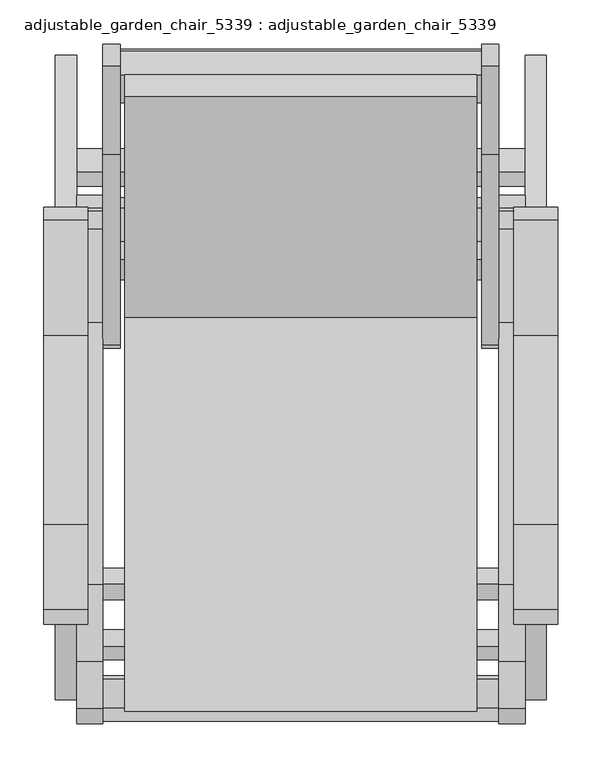
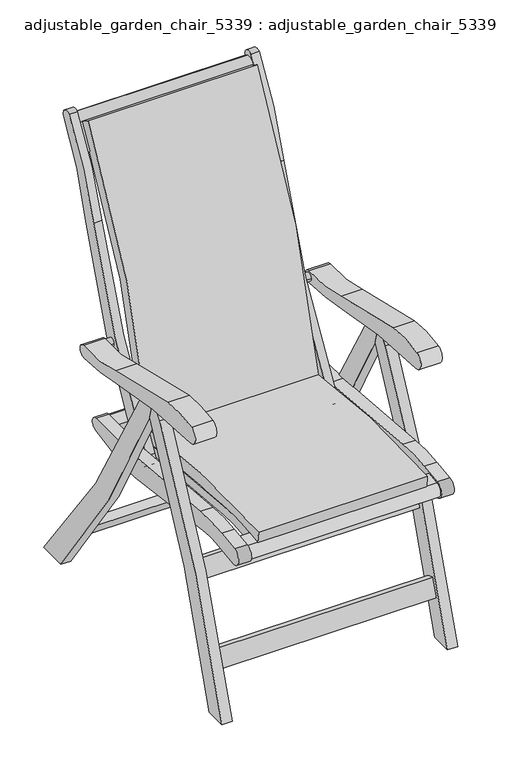
"""IFC4 building model written with IfcOpenShell, lengths in millimetres: furniture geometry, adjustable_garden_chair_5339 : adjustable_garden_chair_5339."""

from ifc_helpers import new_model, si_unit, point, frame, frame_2d, origin, place, context, project, spatial, polyline, circle_curve, trimmed, segment, composite_curve, outline, extrude, source, transform, mapped, element, save


def adjustable_garden_chair_5339_adjustable_garden_chair_5339_e938936b(model_context):
    return source(origin(), model_context, "Body", "SweptSolid", [
        extrude(outline(composite_curve([segment(trimmed(circle_curve(frame_2d((148.1612086, 950.4320275)), 328.1928043), [point((43.4212159, 639.4014009))], [point((175.5033422, 623.3801593))], True, "CARTESIAN"), True, "CONTINUOUS"), segment(trimmed(circle_curve(frame_2d((174.7344479, 608.5698693)), 14.8302356), [point((175.5033422, 623.3801593))], [point((173.9655536, 593.7595793))], False, "CARTESIAN"), True, "CONTINUOUS"), segment(trimmed(circle_curve(frame_2d((181.4513875, 1232.0279279)), 638.3122454), [point((173.9655536, 593.7595793))], [point((39.8991519, 609.6088672))], False, "CARTESIAN"), True, "CONTINUOUS"), segment(trimmed(circle_curve(frame_2d((-275.8190799, -778.6351578)), 1423.692198), [point((39.8991519, 609.6088672))], [point((-263.2618422, 645.0016605))], True, "CARTESIAN"), True, "CONTINUOUS"), segment(trimmed(circle_curve(frame_2d((-263.0738268, 666.3173055)), 21.3164742), [point((-263.2618422, 645.0016605))], [point((-267.5231892, 687.1642537))], False, "CARTESIAN"), True, "CONTINUOUS"), segment(trimmed(circle_curve(frame_2d((-209.9588085, 417.4533248)), 275.7855019), [point((-267.5231892, 687.1642537))], [point((-170.6132595, 690.417738))], False, "CARTESIAN"), True, "CONTINUOUS"), segment(trimmed(circle_curve(frame_2d((-343.645132, -510.0114028)), 1212.8355828), [point((-170.6132595, 690.417738))], [point((43.4212159, 639.4014009))], False, "CARTESIAN"), True, "CONTINUOUS")], self_intersect=False)), frame((242.0, 0.0, 0.0), z_axis=(1.0, 0.0, 0.0), x_axis=(0.0, 1.0, 0.0)), (0.0, 0.0, 1.0), 50.0),
        extrude(outline(composite_curve([segment(trimmed(circle_curve(frame_2d((148.1612086, 950.4320275)), 328.1928043), [point((43.4212159, 639.4014009))], [point((175.5033422, 623.3801593))], True, "CARTESIAN"), True, "CONTINUOUS"), segment(trimmed(circle_curve(frame_2d((174.7344479, 608.5698693)), 14.8302356), [point((175.5033422, 623.3801593))], [point((173.9655536, 593.7595793))], False, "CARTESIAN"), True, "CONTINUOUS"), segment(trimmed(circle_curve(frame_2d((181.4513875, 1232.0279279)), 638.3122454), [point((173.9655536, 593.7595793))], [point((39.8991519, 609.6088672))], False, "CARTESIAN"), True, "CONTINUOUS"), segment(trimmed(circle_curve(frame_2d((-275.8190799, -778.6351578)), 1423.692198), [point((39.8991519, 609.6088672))], [point((-263.2618422, 645.0016605))], True, "CARTESIAN"), True, "CONTINUOUS"), segment(trimmed(circle_curve(frame_2d((-263.0738268, 666.3173055)), 21.3164742), [point((-263.2618422, 645.0016605))], [point((-267.5231892, 687.1642537))], False, "CARTESIAN"), True, "CONTINUOUS"), segment(trimmed(circle_curve(frame_2d((-209.9588085, 417.4533248)), 275.7855019), [point((-267.5231892, 687.1642537))], [point((-170.6132595, 690.417738))], False, "CARTESIAN"), True, "CONTINUOUS"), segment(trimmed(circle_curve(frame_2d((-343.645132, -510.0114028)), 1212.8355828), [point((-170.6132595, 690.417738))], [point((43.4212159, 639.4014009))], False, "CARTESIAN"), True, "CONTINUOUS")], self_intersect=False)), frame((-292.0, 0.0, 0.0), z_axis=(1.0, 0.0, 0.0), x_axis=(0.0, 1.0, 0.0)), (0.0, 0.0, 1.0), 50.0),
        extrude(outline(polyline([(0.0, -20.0), (0.0, 0.0), (295.0, 0.0), (295.0, -20.0), (0.0, -20.0)])), frame((147.5, 137.5882722, 568.6800749), z_axis=(0.0, 0.2533030270582979, 0.9673869838296892), x_axis=(-1.0, 0.0, 0.0)), (0.0, 0.0, 1.0), 20.0),
        extrude(outline(polyline([(0.0, -20.0), (0.0, 0.0), (295.0, 0.0), (295.0, -20.0), (0.0, -20.0)])), frame((147.5, 147.2074959, 603.5678435), z_axis=(0.0, 0.2719015325291372, 0.9623250784471465), x_axis=(-1.0, 0.0, 0.0)), (0.0, 0.0, 1.0), 20.0),
        extrude(outline(polyline([(0.0, -19.9999999), (0.0, 0.0), (295.0, 0.0), (295.0, -19.9999999), (0.0, -19.9999999)])), frame((147.5, 157.4973647, 638.2637288), z_axis=(0.0, 0.2903990191599495, 0.9569056430343272), x_axis=(-1.0, 0.0, 0.0)), (0.0, 0.0, 1.0), 20.0),
        extrude(outline(polyline([(0.0, -20.0000001), (0.0, 0.0), (295.0, 0.0), (295.0, -20.0000001), (0.0, -20.0000001)])), frame((147.5, 168.4540556, 672.7548405), z_axis=(0.0, 0.30878861462961876, 0.9511306910593943), x_axis=(-1.0, 0.0, 0.0)), (0.0, 0.0, 1.0), 20.0),
        extrude(outline(polyline([(0.0, -20.0), (0.0, 0.0), (295.0, 0.0), (295.0, -20.0), (0.0, -20.0)])), frame((147.5, 180.073498, 707.028364), z_axis=(0.0, 0.3270634867015429, 0.9450023680746149), x_axis=(-1.0, 0.0, 0.0)), (0.0, 0.0, 1.0), 20.0),
        extrude(outline(polyline([(0.0, -20.0), (0.0, 0.0), (295.0, 0.0), (295.0, -20.0), (0.0, -20.0)])), frame((147.5, 192.3513749, 741.071566), z_axis=(0.0, 0.3452168457619835, 0.9385229509192341), x_axis=(-1.0, 0.0, 0.0)), (0.0, 0.0, 1.0), 20.0),
        extrude(outline(polyline([(0.0, -20.0), (0.0, 0.0), (295.0, 0.0), (295.0, -20.0), (0.0, -20.0)])), frame((147.5, 205.2831247, 774.8717983), z_axis=(0.0, 0.3632419473426192, 0.9316948468735576), x_axis=(-1.0, 0.0, 0.0)), (0.0, 0.0, 1.0), 20.0),
        extrude(outline(polyline([(0.0, -20.0), (0.0, 0.0), (295.0, 0.0), (295.0, -20.0), (0.0, -20.0)])), frame((147.5, 218.863943, 808.4165033), z_axis=(0.0, 0.38113209462627146, 0.9245205927645911), x_axis=(-1.0, 0.0, 0.0)), (0.0, 0.0, 1.0), 20.0),
        extrude(outline(polyline([(0.0, -20.0000001), (0.0, 0.0), (295.0, 0.0), (295.0, -20.0000001), (0.0, -20.0000001)])), frame((147.5, 233.088784, 841.6932183), z_axis=(0.0, 0.39888064093497316, 0.9170028540235331), x_axis=(-1.0, 0.0, 0.0)), (0.0, 0.0, 1.0), 20.0),
        extrude(outline(polyline([(0.0, -20.0), (0.0, 0.0), (295.0, 0.0), (295.0, -20.0), (0.0, -20.0)])), frame((147.5, 244.4121321, 867.0975304), z_axis=(0.0, 0.4164809921993657, 0.9091444236955051), x_axis=(-1.0, 0.0, 0.0)), (0.0, 0.0, 1.0), 20.0),
        extrude(outline(polyline([(0.0, -20.0), (0.0, 0.0), (295.0, 0.0), (295.0, -20.0), (0.0, -20.0)])), frame((147.5, 259.9089267, 899.8012797), z_axis=(0.0, 0.43392660940863675, 0.9009482214018321), x_axis=(-1.0, 0.0, 0.0)), (0.0, 0.0, 1.0), 20.0),
        extrude(outline(polyline([(0.0, -20.0000001), (0.0, 0.0), (295.0, 0.0), (295.0, -20.0000001), (0.0, -20.0000001)])), frame((147.5, 276.0331794, 932.2002663), z_axis=(0.0, 0.4512110110398427, 0.892417292255368), x_axis=(-1.0, 0.0, 0.0)), (0.0, 0.0, 1.0), 20.0),
        extrude(outline(polyline([(0.0, -20.0), (0.0, 0.0), (295.0, 0.0), (295.0, -20.0), (0.0, -20.0)])), frame((147.5, 292.7788997, 964.2824531), z_axis=(0.0, 0.4683277754660565, 0.8835548057291156), x_axis=(-1.0, 0.0, 0.0)), (0.0, 0.0, 1.0), 20.0),
        extrude(outline(composite_curve([segment(polyline([(150.6635772, 538.0199468), (130.6557697, 548.6582867)]), True, "CONTINUOUS"), segment(trimmed(circle_curve(frame_2d((1820.3447932, 139.3902819)), 1738.5480424), [point((130.6557697, 548.6582867))], [point((311.3178699, 1002.7482844))], False, "CARTESIAN"), True, "CONTINUOUS"), segment(polyline([(311.3178699, 1002.7482844), (330.8196286, 992.6521155)]), True, "CONTINUOUS"), segment(trimmed(circle_curve(frame_2d((1820.3447932, 139.3902819)), 1716.607402), [point((330.8196286, 992.6521155))], [point((150.6635772, 538.0199468))], True, "CARTESIAN"), True, "CONTINUOUS")], self_intersect=False)), frame((147.5, 0.0, 0.0), z_axis=(1.0, 0.0, 0.0), x_axis=(0.0, 1.0, 0.0)), (0.0, 0.0, 1.0), 32.5),
        extrude(outline(composite_curve([segment(polyline([(150.6635772, 538.0199468), (130.6557697, 548.6582867)]), True, "CONTINUOUS"), segment(trimmed(circle_curve(frame_2d((1820.3447932, 139.3902819)), 1738.5480424), [point((130.6557697, 548.6582867))], [point((311.3178699, 1002.7482844))], False, "CARTESIAN"), True, "CONTINUOUS"), segment(polyline([(311.3178699, 1002.7482844), (330.8196286, 992.6521155)]), True, "CONTINUOUS"), segment(trimmed(circle_curve(frame_2d((1820.3447932, 139.3902819)), 1716.607402), [point((330.8196286, 992.6521155))], [point((150.6635772, 538.0199468))], True, "CARTESIAN"), True, "CONTINUOUS")], self_intersect=False)), frame((-180.0, 0.0, 0.0), z_axis=(1.0, 0.0, 0.0), x_axis=(0.0, 1.0, 0.0)), (0.0, 0.0, 1.0), 32.5),
        extrude(outline(polyline([(0.0, -22.0), (0.0, 0.0), (411.0, 0.0), (411.0, -22.0), (0.0, -22.0)])), frame((205.5, 107.1821916, 504.5109071), z_axis=(0.0, 0.46947156278588487, 0.8829475928589302), x_axis=(-1.0, 0.0, 0.0)), (0.0, 0.0, 1.0), 50.0),
        extrude(outline(composite_curve([segment(polyline([(369.2008252, 1058.8126612), (327.1980391, 984.9156655), (308.0717579, 995.7869748), (340.1915354, 1052.2964421)]), True, "CONTINUOUS"), segment(trimmed(circle_curve(frame_2d((357.5790638, 1042.4134336)), 20.0), [point((340.1915354, 1052.2964421))], [point((367.4620723, 1059.800962))], False, "CARTESIAN"), True, "CONTINUOUS"), segment(polyline([(367.4620723, 1059.800962), (369.2008252, 1058.8126612)]), True, "CONTINUOUS")], self_intersect=False)), frame((-205.5, 0.0, 0.0), z_axis=(1.0, 0.0, 0.0), x_axis=(0.0, 1.0, 0.0)), (0.0, 0.0, 1.0), 411.0),
        extrude(outline(composite_curve([segment(trimmed(circle_curve(frame_2d((-1314.5285091, 1298.2546646)), 1660.3335522), [point((284.5644955, 851.478359))], [point((71.610087, 384.292249))], False, "CARTESIAN"), True, "CONTINUOUS"), segment(trimmed(circle_curve(frame_2d((52.4582417, 396.9808098)), 22.9737405), [point((71.610087, 384.292249))], [point((33.307137, 409.6704883))], False, "CARTESIAN"), True, "CONTINUOUS"), segment(trimmed(circle_curve(frame_2d((-1197.5178376, 1277.8037867)), 1506.1824398), [point((33.307137, 409.6704883))], [point((249.8732333, 861.0968995))], True, "CARTESIAN"), True, "CONTINUOUS"), segment(trimmed(circle_curve(frame_2d((939.3593126, 662.5924291)), 717.4922148), [point((249.8732333, 861.0968995))], [point((350.3591165, 1072.3165403))], False, "CARTESIAN"), True, "CONTINUOUS"), segment(trimmed(circle_curve(frame_2d((359.5368178, 1059.9113552)), 15.4310991), [point((350.3591165, 1072.3165403))], [point((374.7410315, 1057.2749365))], False, "CARTESIAN"), True, "CONTINUOUS"), segment(trimmed(circle_curve(frame_2d((878.1941568, 714.0152031)), 609.3375862), [point((374.7410315, 1057.2749365))], [point((284.5644955, 851.478359))], True, "CARTESIAN"), True, "CONTINUOUS")], self_intersect=False)), frame((205.5, 0.0, 0.0), z_axis=(1.0, 0.0, 0.0), x_axis=(0.0, 1.0, 0.0)), (0.0, 0.0, 1.0), 19.5),
        extrude(outline(composite_curve([segment(trimmed(circle_curve(frame_2d((-1314.5305815, 1298.2556309)), 1660.3358082), [point((284.5644955, 851.478359))], [point((71.6100814, 384.2922516))], False, "CARTESIAN"), True, "CONTINUOUS"), segment(trimmed(circle_curve(frame_2d((52.4582393, 396.9808109)), 22.973737), [point((71.6100814, 384.2922516))], [point((33.3071379, 409.6704879))], False, "CARTESIAN"), True, "CONTINUOUS"), segment(trimmed(circle_curve(frame_2d((-1197.5180648, 1277.8038927)), 1506.1826875), [point((33.3071379, 409.6704879))], [point((249.8732333, 861.0968995))], True, "CARTESIAN"), True, "CONTINUOUS"), segment(trimmed(circle_curve(frame_2d((939.3594209, 662.5923787)), 717.4923328), [point((249.8732333, 861.0968995))], [point((350.3591359, 1072.3165688))], False, "CARTESIAN"), True, "CONTINUOUS"), segment(trimmed(circle_curve(frame_2d((359.53684, 1059.9114029)), 15.4310853), [point((350.3591359, 1072.3165688))], [point((374.7410315, 1057.2749365))], False, "CARTESIAN"), True, "CONTINUOUS"), segment(trimmed(circle_curve(frame_2d((878.1941568, 714.0152031)), 609.3375862), [point((374.7410315, 1057.2749365))], [point((284.5644955, 851.478359))], True, "CARTESIAN"), True, "CONTINUOUS")], self_intersect=False)), frame((-225.0, 0.0, 0.0), z_axis=(1.0, 0.0, 0.0), x_axis=(0.0, 1.0, 0.0)), (0.0, 0.0, 1.0), 19.5),
        extrude(outline(composite_curve([segment(polyline([(-83.9411598, 628.8858688), (-73.4314655, 590.0)]), True, "CONTINUOUS"), segment(trimmed(circle_curve(frame_2d((2150.5800409, -679.3988459)), 2560.78125), [point((-73.4314655, 590.0))], [point((-318.4314655, 0.0))], True, "CARTESIAN"), True, "CONTINUOUS"), segment(polyline([(-318.4314655, 0.0), (-370.0, 0.0)]), True, "CONTINUOUS"), segment(trimmed(circle_curve(frame_2d((2141.3775013, -695.7889548)), 2605.9814319), [point((-370.0, 0.0))], [point((-115.5965217, 606.9802048))], False, "CARTESIAN"), True, "CONTINUOUS"), segment(trimmed(circle_curve(frame_2d((-73.4314655, 579.8735129)), 50.1264871), [point((-115.5965217, 606.9802048))], [point((-83.9411598, 628.8858688))], False, "CARTESIAN"), True, "CONTINUOUS")], self_intersect=False)), frame((255.0, 0.0, 0.0), z_axis=(1.0, 0.0, 0.0), x_axis=(0.0, 1.0, 0.0)), (0.0, 0.0, 1.0), 24.0),
        extrude(outline(composite_curve([segment(polyline([(362.21428, 0.0), (291.5685345, 0.0)]), True, "CONTINUOUS"), segment(trimmed(circle_curve(frame_2d((2658.8629803, 1872.415208)), 3018.28125), [point((291.5685345, 0.0))], [point((-73.4314655, 590.0))], False, "CARTESIAN"), True, "CONTINUOUS"), segment(polyline([(-73.4314655, 590.0), (-83.9411598, 628.8858688)]), True, "CONTINUOUS"), segment(trimmed(circle_curve(frame_2d((-72.4622197, 583.5932512)), 46.7245896), [point((-83.9411598, 628.8858688))], [point((-30.5273572, 604.2004001))], False, "CARTESIAN"), True, "CONTINUOUS"), segment(trimmed(circle_curve(frame_2d((2678.9114955, 1935.6417432)), 3018.90625), [point((-30.5273572, 604.2004001))], [point((362.21428, 0.0))], True, "CARTESIAN"), True, "CONTINUOUS")], self_intersect=False)), frame((255.0, 0.0, 0.0), z_axis=(1.0, 0.0, 0.0), x_axis=(0.0, 1.0, 0.0)), (0.0, 0.0, 1.0), 24.0),
        extrude(outline(composite_curve([segment(polyline([(-83.9411598, 628.8858688), (-73.4314655, 590.0)]), True, "CONTINUOUS"), segment(trimmed(circle_curve(frame_2d((2150.5800409, -679.3988459)), 2560.78125), [point((-73.4314655, 590.0))], [point((-318.4314655, 0.0))], True, "CARTESIAN"), True, "CONTINUOUS"), segment(polyline([(-318.4314655, 0.0), (-370.0, 0.0)]), True, "CONTINUOUS"), segment(trimmed(circle_curve(frame_2d((2141.3775013, -695.7889548)), 2605.9814319), [point((-370.0, 0.0))], [point((-115.5965217, 606.9802048))], False, "CARTESIAN"), True, "CONTINUOUS"), segment(trimmed(circle_curve(frame_2d((-73.4314655, 579.8735129)), 50.1264871), [point((-115.5965217, 606.9802048))], [point((-83.9411598, 628.8858688))], False, "CARTESIAN"), True, "CONTINUOUS")], self_intersect=False)), frame((-279.0, 0.0, 0.0), z_axis=(1.0, 0.0, 0.0), x_axis=(0.0, 1.0, 0.0)), (0.0, 0.0, 1.0), 24.0),
        extrude(outline(composite_curve([segment(polyline([(362.21428, 0.0), (291.5685345, 0.0)]), True, "CONTINUOUS"), segment(trimmed(circle_curve(frame_2d((2658.8629803, 1872.415208)), 3018.28125), [point((291.5685345, 0.0))], [point((-73.4314655, 590.0))], False, "CARTESIAN"), True, "CONTINUOUS"), segment(polyline([(-73.4314655, 590.0), (-83.9411598, 628.8858688)]), True, "CONTINUOUS"), segment(trimmed(circle_curve(frame_2d((-72.4622197, 583.5932512)), 46.7245896), [point((-83.9411598, 628.8858688))], [point((-30.5273572, 604.2004001))], False, "CARTESIAN"), True, "CONTINUOUS"), segment(trimmed(circle_curve(frame_2d((2678.9114955, 1935.6417432)), 3018.90625), [point((-30.5273572, 604.2004001))], [point((362.21428, 0.0))], True, "CARTESIAN"), True, "CONTINUOUS")], self_intersect=False)), frame((-279.0, 0.0, 0.0), z_axis=(1.0, 0.0, 0.0), x_axis=(0.0, 1.0, 0.0)), (0.0, 0.0, 1.0), 24.0),
        extrude(outline(composite_curve([segment(polyline([(-238.8791572, 446.1253746), (58.4788796, 420.0), (188.2161711, 420.0)]), True, "CONTINUOUS"), segment(trimmed(circle_curve(frame_2d((188.2161711, 405.0)), 15.0), [point((188.2161711, 420.0))], [point((191.0033734, 390.2612245))], False, "CARTESIAN"), True, "CONTINUOUS"), segment(polyline([(191.0033734, 390.2612245), (86.6960303, 370.5359993)]), True, "CONTINUOUS"), segment(trimmed(circle_curve(frame_2d((53.2496027, 547.4013053)), 180.0), [point((86.6960303, 370.5359993))], [point((30.0021337, 368.908854))], False, "CARTESIAN"), True, "CONTINUOUS"), segment(polyline([(30.0021337, 368.908854), (-260.5570748, 406.7522817)]), True, "CONTINUOUS"), segment(trimmed(circle_curve(frame_2d((-283.1587807, 233.217954)), 175.0), [point((-260.5570748, 406.7522817))], [point((-305.4087938, 406.7977251))], True, "CARTESIAN"), True, "CONTINUOUS"), segment(polyline([(-305.4087938, 406.7977251), (-375.0765946, 397.8674824)]), True, "CONTINUOUS"), segment(trimmed(circle_curve(frame_2d((-377.6194532, 417.7051705)), 20.0), [point((-375.0765946, 397.8674824))], [point((-380.1623119, 437.5428586))], False, "CARTESIAN"), True, "CONTINUOUS"), segment(polyline([(-380.1623119, 437.5428586), (-326.8914381, 444.3712905)]), True, "CONTINUOUS"), segment(trimmed(circle_curve(frame_2d((-274.7628361, 37.698684)), 410.0), [point((-326.8914381, 444.3712905))], [point((-238.8791572, 446.1253746))], False, "CARTESIAN"), True, "CONTINUOUS")], self_intersect=False)), frame((225.0, 0.0, 0.0), z_axis=(1.0, 0.0, 0.0), x_axis=(0.0, 1.0, 0.0)), (0.0, 0.0, 1.0), 30.0),
        extrude(outline(composite_curve([segment(polyline([(-238.8791572, 446.1253746), (58.4788796, 420.0), (188.2161711, 420.0)]), True, "CONTINUOUS"), segment(trimmed(circle_curve(frame_2d((188.2161711, 405.0)), 15.0), [point((188.2161711, 420.0))], [point((191.0033734, 390.2612245))], False, "CARTESIAN"), True, "CONTINUOUS"), segment(polyline([(191.0033734, 390.2612245), (86.6960303, 370.5359993)]), True, "CONTINUOUS"), segment(trimmed(circle_curve(frame_2d((53.2496027, 547.4013053)), 180.0), [point((86.6960303, 370.5359993))], [point((30.0021337, 368.908854))], False, "CARTESIAN"), True, "CONTINUOUS"), segment(polyline([(30.0021337, 368.908854), (-260.5570748, 406.7522817)]), True, "CONTINUOUS"), segment(trimmed(circle_curve(frame_2d((-283.1587807, 233.217954)), 175.0), [point((-260.5570748, 406.7522817))], [point((-305.4087938, 406.7977251))], True, "CARTESIAN"), True, "CONTINUOUS"), segment(polyline([(-305.4087938, 406.7977251), (-375.0765946, 397.8674824)]), True, "CONTINUOUS"), segment(trimmed(circle_curve(frame_2d((-377.6194532, 417.7051705)), 20.0), [point((-375.0765946, 397.8674824))], [point((-380.1623119, 437.5428586))], False, "CARTESIAN"), True, "CONTINUOUS"), segment(polyline([(-380.1623119, 437.5428586), (-326.8914381, 444.3712905)]), True, "CONTINUOUS"), segment(trimmed(circle_curve(frame_2d((-274.7628361, 37.698684)), 410.0), [point((-326.8914381, 444.3712905))], [point((-238.8791572, 446.1253746))], False, "CARTESIAN"), True, "CONTINUOUS")], self_intersect=False)), frame((-255.0, 0.0, 0.0), z_axis=(1.0, 0.0, 0.0), x_axis=(0.0, 1.0, 0.0)), (0.0, 0.0, 1.0), 30.0),
        extrude(outline(composite_curve([segment(polyline([(-379.7808831, 434.5672054), (-347.0486977, 438.7629222), (-342.725838, 405.0388524), (-375.4580234, 400.8431356)]), True, "CONTINUOUS"), segment(trimmed(circle_curve(frame_2d((-377.6194532, 417.7051705)), 17.0), [point((-375.4580234, 400.8431356))], [point((-379.7808831, 434.5672054))], False, "CARTESIAN"), True, "CONTINUOUS")], self_intersect=False)), frame((-225.0, 0.0, 0.0), z_axis=(1.0, 0.0, 0.0), x_axis=(0.0, 1.0, 0.0)), (0.0, 0.0, 1.0), 450.0),
        extrude(outline(composite_curve([segment(trimmed(circle_curve(frame_2d((188.2161711, 404.8670728)), 12.1329272), [point((188.2161711, 417.0))], [point((188.2161711, 392.7341457))], False, "CARTESIAN"), True, "CONTINUOUS"), segment(polyline([(188.2161711, 392.7341457), (150.2161711, 392.7341457), (150.2161711, 417.0), (188.2161711, 417.0)]), True, "CONTINUOUS")], self_intersect=False)), frame((-225.0, 0.0, 0.0), z_axis=(1.0, 0.0, 0.0), x_axis=(0.0, 1.0, 0.0)), (0.0, 0.0, 1.0), 450.0),
        extrude(outline(composite_curve([segment(polyline([(58.2596561, 415.0), (150.2161711, 415.0), (150.2161711, 393.0), (57.2950725, 393.0), (-241.2422287, 419.2289828)]), True, "CONTINUOUS"), segment(trimmed(circle_curve(frame_2d((-274.7628361, 37.698684)), 383.0), [point((-241.2422287, 419.2289828))], [point((-323.4585789, 417.5904115))], True, "CARTESIAN"), True, "CONTINUOUS"), segment(polyline([(-323.4585789, 417.5904115), (-343.9972673, 414.9576964), (-346.7944118, 436.7791534), (-326.2557234, 439.4118685)]), True, "CONTINUOUS"), segment(trimmed(circle_curve(frame_2d((-274.7628361, 37.698684)), 405.0), [point((-326.2557234, 439.4118685))], [point((-239.3167631, 441.1445613))], False, "CARTESIAN"), True, "CONTINUOUS"), segment(polyline([(-239.3167631, 441.1445613), (58.2596561, 415.0)]), True, "CONTINUOUS")], self_intersect=False)), frame((-200.0, 0.0, 0.0), z_axis=(1.0, 0.0, 0.0), x_axis=(0.0, 1.0, 0.0)), (0.0, 0.0, 1.0), 35.0),
        extrude(outline(composite_curve([segment(polyline([(58.2596561, 415.0), (150.2161711, 415.0), (150.2161711, 393.0), (57.2950725, 393.0), (-241.2422287, 419.2289828)]), True, "CONTINUOUS"), segment(trimmed(circle_curve(frame_2d((-274.7628361, 37.698684)), 383.0), [point((-241.2422287, 419.2289828))], [point((-323.4585789, 417.5904115))], True, "CARTESIAN"), True, "CONTINUOUS"), segment(polyline([(-323.4585789, 417.5904115), (-343.9972673, 414.9576964), (-346.7944118, 436.7791534), (-326.2557234, 439.4118685)]), True, "CONTINUOUS"), segment(trimmed(circle_curve(frame_2d((-274.7628361, 37.698684)), 405.0), [point((-326.2557234, 439.4118685))], [point((-239.3167631, 441.1445613))], False, "CARTESIAN"), True, "CONTINUOUS"), segment(polyline([(-239.3167631, 441.1445613), (58.2596561, 415.0)]), True, "CONTINUOUS")], self_intersect=False)), frame((165.0, 0.0, 0.0), z_axis=(1.0, 0.0, 0.0), x_axis=(0.0, 1.0, 0.0)), (0.0, 0.0, 1.0), 35.0),
        extrude(outline(polyline([(0.0, -20.0), (0.0, 0.0), (330.0, 0.0), (330.0, -20.0), (0.0, -20.0)])), frame((165.0, -329.8129674, 417.7918808), z_axis=(0.0, -0.10015135080024025, 0.9949722141511729), x_axis=(-1.0, 0.0, 0.0)), (0.0, 0.0, 1.0), 20.0),
        extrude(outline(polyline([(0.0, -20.0), (0.0, 0.0), (330.0, 0.0), (330.0, -20.0), (0.0, -20.0)])), frame((165.0, -295.940466, 420.5485593), z_axis=(0.0, -0.05430307370314669, 0.9985244995423951), x_axis=(-1.0, 0.0, 0.0)), (0.0, 0.0, 1.0), 20.0),
        extrude(outline(polyline([(0.0, -20.0), (0.0, 0.0), (330.0, 0.0), (330.0, -20.0), (0.0, -20.0)])), frame((165.0, -262.8732701, 420.9868234), z_axis=(0.0, 0.0399406917008388, 0.9992020522128938), x_axis=(-1.0, 0.0, 0.0)), (0.0, 0.0, 1.0), 20.0),
        extrude(outline(polyline([(0.0, -19.9999999), (0.0, 0.0), (330.0, 0.0), (330.0, -19.9999999), (0.0, -19.9999999)])), frame((165.0, -228.8710651, 419.149381), z_axis=(0.0, 0.0862771077257393, 0.9962711782855516), x_axis=(-1.0, 0.0, 0.0)), (0.0, 0.0, 1.0), 20.0),
        extrude(outline(polyline([(0.0, -19.9999999), (0.0, 0.0), (330.0, 0.0), (330.0, -19.9999999), (0.0, -19.9999999)])), frame((165.0, -194.005372, 416.0861402), z_axis=(0.0, 0.0862771077257393, 0.9962711782855516), x_axis=(-1.0, 0.0, 0.0)), (0.0, 0.0, 1.0), 20.0),
        extrude(outline(polyline([(0.0, -19.9999999), (0.0, 0.0), (330.0, 0.0), (330.0, -19.9999999), (0.0, -19.9999999)])), frame((165.0, -159.1396789, 413.0228993), z_axis=(0.0, 0.08627710772573936, 0.9962711782855516), x_axis=(-1.0, 0.0, 0.0)), (0.0, 0.0, 1.0), 20.0),
        extrude(outline(polyline([(0.0, -19.9999999), (0.0, 0.0), (330.0, 0.0), (330.0, -19.9999999), (0.0, -19.9999999)])), frame((165.0, -124.2739858, 409.9596584), z_axis=(0.0, 0.08627710772573943, 0.9962711782855516), x_axis=(-1.0, 0.0, 0.0)), (0.0, 0.0, 1.0), 20.0),
        extrude(outline(polyline([(0.0, -19.9999999), (0.0, 0.0), (330.0, 0.0), (330.0, -19.9999999), (0.0, -19.9999999)])), frame((165.0, -89.4082927, 406.8964175), z_axis=(0.0, 0.0862771077257394, 0.9962711782855516), x_axis=(-1.0, 0.0, 0.0)), (0.0, 0.0, 1.0), 20.0),
        extrude(outline(polyline([(0.0, -19.9999999), (0.0, 0.0), (330.0, 0.0), (330.0, -19.9999999), (0.0, -19.9999999)])), frame((165.0, -54.5425996, 403.8331766), z_axis=(0.0, 0.0862771077257394, 0.9962711782855516), x_axis=(-1.0, 0.0, 0.0)), (0.0, 0.0, 1.0), 20.0),
        extrude(outline(polyline([(0.0, -19.9999999), (0.0, 0.0), (330.0, 0.0), (330.0, -19.9999999), (0.0, -19.9999999)])), frame((165.0, -19.6769065, 400.7699358), z_axis=(0.0, 0.08627710772573942, 0.9962711782855516), x_axis=(-1.0, 0.0, 0.0)), (0.0, 0.0, 1.0), 20.0),
        extrude(outline(polyline([(0.0, -19.9999999), (0.0, 0.0), (330.0, 0.0), (330.0, -19.9999999), (0.0, -19.9999999)])), frame((165.0, 15.1887866, 397.7066949), z_axis=(0.0, 0.0862771077257394, 0.9962711782855516), x_axis=(-1.0, 0.0, 0.0)), (0.0, 0.0, 1.0), 20.0),
        extrude(outline(polyline([(0.0, -20.0), (0.0, 0.0), (330.0, 0.0), (330.0, -20.0), (0.0, -20.0)])), frame((165.0, 50.5659752, 394.1151581), z_axis=(0.0, 0.03230033547544253, 0.9994782080306573), x_axis=(-1.0, 0.0, 0.0)), (0.0, 0.0, 1.0), 20.0),
        extrude(outline(polyline([(165.0, 106.2119819), (165.0, 86.2119819), (-165.0, 86.2119819), (-165.0, 106.2119819), (165.0, 106.2119819)])), frame((0.0, 0.0, 394.1047223), z_axis=(0.0, 0.0, 1.0), x_axis=(1.0, 0.0, 0.0)), (0.0, 0.0, 1.0), 20.0),
        extrude(outline(polyline([(165.0, 141.2119819), (165.0, 121.2119819), (-165.0, 121.2119819), (-165.0, 141.2119819), (165.0, 141.2119819)])), frame((0.0, 0.0, 394.1047223), z_axis=(0.0, 0.0, 1.0), x_axis=(1.0, 0.0, 0.0)), (0.0, 0.0, 1.0), 20.0),
        extrude(outline(polyline([(0.0, -20.0), (0.0, 0.0), (510.0, 0.0), (510.0, -20.0), (0.0, -20.0)])), frame((255.0, -324.5742376, 103.4202014), z_axis=(0.0, 0.34202014332566577, 0.9396926207859095), x_axis=(-1.0, 0.0, 0.0)), (0.0, 0.0, 1.0), 45.0),
        extrude(outline(polyline([(0.0, -20.0), (0.0, 0.0), (510.0, 0.0), (510.0, -20.0), (0.0, -20.0)])), frame((255.0, 239.7030548, 94.1221475), z_axis=(0.0, -0.5877852522924797, 0.8090169943749427), x_axis=(-1.0, 0.0, 0.0)), (0.0, 0.0, 1.0), 45.0),
        extrude(outline(polyline([(0.0, -20.0), (0.0, 0.0), (510.0, 0.0), (510.0, -20.0), (0.0, -20.0)])), frame((255.0, -256.6989851, 287.857913), z_axis=(0.0, 0.3907311284892644, 0.9205048534524444), x_axis=(-1.0, 0.0, 0.0)), (0.0, 0.0, 1.0), 45.0),
        extrude(outline(composite_curve([segment(trimmed(circle_curve(frame_2d((175.2156419, 609.0447403)), 10.0), [point((165.2603514, 609.9892995))], [point((185.1709323, 608.1001811))], False, "CARTESIAN"), True, "CONTINUOUS"), segment(trimmed(circle_curve(frame_2d((175.2156419, 609.0447403)), 10.0), [point((185.1709323, 608.1001811))], [point((165.2603514, 609.9892995))], False, "CARTESIAN"), True, "CONTINUOUS")], self_intersect=False)), frame((-242.0, 0.0, 0.0), z_axis=(1.0, 0.0, 0.0), x_axis=(0.0, 1.0, 0.0)), (0.0, 0.0, 1.0), 17.0),
        extrude(outline(composite_curve([segment(trimmed(circle_curve(frame_2d((175.2156419, 609.0447403)), 10.0), [point((165.2603514, 609.9892995))], [point((185.1709323, 608.1001811))], False, "CARTESIAN"), True, "CONTINUOUS"), segment(trimmed(circle_curve(frame_2d((175.2156419, 609.0447403)), 10.0), [point((185.1709323, 608.1001811))], [point((165.2603514, 609.9892995))], False, "CARTESIAN"), True, "CONTINUOUS")], self_intersect=False)), frame((225.0, 0.0, 0.0), z_axis=(1.0, 0.0, 0.0), x_axis=(0.0, 1.0, 0.0)), (0.0, 0.0, 1.0), 17.0),
        extrude(outline(composite_curve([segment(trimmed(circle_curve(frame_2d((-231.1593215, -1529.137865)), 1967.2571003), [point((83.6234956, 412.7715759))], [point((-380.8093658, 432.4190072))], True, "CARTESIAN"), True, "CONTINUOUS"), segment(polyline([(-380.8093658, 432.4190072), (-383.0914779, 462.3320807)]), True, "CONTINUOUS"), segment(trimmed(circle_curve(frame_2d((-231.1593215, -1529.137865)), 1997.2571003), [point((-383.0914779, 462.3320807))], [point((88.4238262, 442.3850328))], False, "CARTESIAN"), True, "CONTINUOUS"), segment(polyline([(88.4238262, 442.3850328), (83.6234956, 412.7715759)]), True, "CONTINUOUS")], self_intersect=False)), frame((-200.0, 0.0, 0.0), z_axis=(1.0, 0.0, 0.0), x_axis=(0.0, 1.0, 0.0)), (0.0, 0.0, 1.0), 400.0),
        extrude(outline(composite_curve([segment(trimmed(circle_curve(frame_2d((1798.4338397, 104.7835367)), 1738.5480424), [point((340.9641484, 1052.5869946))], [point((89.7658108, 425.7241274))], True, "CARTESIAN"), True, "CONTINUOUS"), segment(polyline([(89.7658108, 425.7241274), (60.2814137, 431.2622072)]), True, "CONTINUOUS"), segment(trimmed(circle_curve(frame_2d((1798.4338397, 104.7835367)), 1768.5480424), [point((60.2814137, 431.2622072))], [point((315.8143742, 1068.9420811))], False, "CARTESIAN"), True, "CONTINUOUS"), segment(polyline([(315.8143742, 1068.9420811), (340.9641484, 1052.5869946)]), True, "CONTINUOUS")], self_intersect=False)), frame((-200.0, 0.0, 0.0), z_axis=(1.0, 0.0, 0.0), x_axis=(0.0, 1.0, 0.0)), (0.0, 0.0, 1.0), 400.0),
    ])


if __name__ == "__main__":
    model = new_model("IFC4")
    model_context = context("Model", 3, world=origin())
    ifc_project = project(units=[si_unit("LENGTHUNIT", "METRE", prefix="MILLI")], contexts=[model_context])
    site = spatial("IfcSite", under=ifc_project)
    building = spatial("IfcBuilding", under=site)
    placement = place(None, origin())
    adjustable_garden_chair_5339_adjustable_garden_chair_5339_shape = adjustable_garden_chair_5339_adjustable_garden_chair_5339_e938936b(model_context)
    element("IfcFurniture", 1, ObjectType="adjustable_garden_chair_5339 : adjustable_garden_chair_5339", at=placement, inside=building, context=model_context, shape_type="MappedRepresentation", body=[
        mapped(adjustable_garden_chair_5339_adjustable_garden_chair_5339_shape, transform((0.0, 0.0, 0.0), x_axis=(1.0, 0.0, 0.0), y_axis=(0.0, 1.0, 0.0), z_axis=(0.0, 0.0, 1.0))),
    ])
    save(model, "model.ifc")

# Revit data of these elements
# Type "adjustable_garden_chair_5339 : adjustable_garden_chair_5339"
#   URL = "www.revitlog.nl"
#   diepte = 2' - 7.49606"
#   corner back [instance default] = 120.00°
#   breedte = 1' - 8.07874"
#   kussen visible [instance default] = yes
#   stoel = hout
#   Default Elevation = 0
# Element 1 (IfcFurniture, "adjustable_garden_chair_5339 : adjustable_garden_chair_5339")
#   Materials on its faces: "hout"
# Materials
#   "hout": class "Wood", colour RGB 140 61 26, transparency 0
